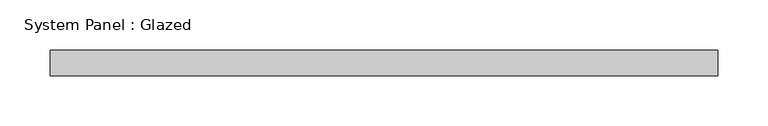
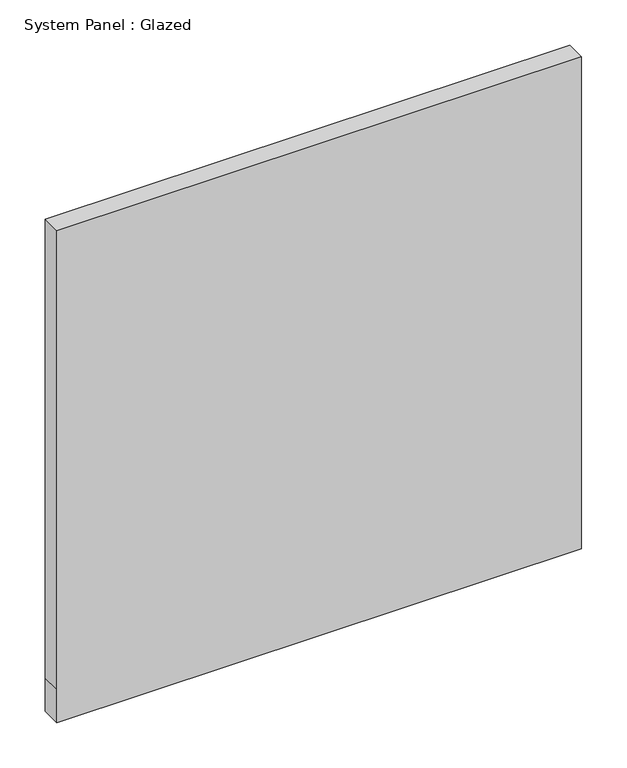
"""IFC4 building model written with IfcOpenShell, lengths in millimetres: plate geometry, System Panel : Glazed."""

from ifc_helpers import new_model, si_unit, frame, origin, place, context, project, spatial, polyline, outline, extrude, source, transform, mapped, element, save


def system_panel_glazed_81358e4c(model_context):
    return source(origin(), model_context, "Body", "SweptSolid", [
        extrude(outline(polyline([(0.0, -333.375), (0.0, 333.375), (44.45, 333.375), (660.9888769, 333.375), (660.9888769, -333.375), (44.45, -333.375), (0.0, -333.375)])), frame((0.0, 19.05, 0.0), z_axis=(0.0, 1.0, 0.0), x_axis=(0.0, 0.0, 1.0)), (0.0, 0.0, 1.0), 25.4),
    ])


if __name__ == "__main__":
    model = new_model("IFC4")
    model_context = context("Model", 3, world=origin())
    ifc_project = project(units=[si_unit("LENGTHUNIT", "METRE", prefix="MILLI")], contexts=[model_context])
    site = spatial("IfcSite", under=ifc_project)
    building = spatial("IfcBuilding", under=site)
    placement = place(None, origin())
    system_panel_glazed_shape = system_panel_glazed_81358e4c(model_context)
    element("IfcPlate", 1, ObjectType="System Panel : Glazed", at=placement, inside=building, context=model_context, shape_type="MappedRepresentation", body=[
        mapped(system_panel_glazed_shape, transform((0.0, 0.0, 0.0), x_axis=(1.0, 0.0, 0.0), y_axis=(0.0, 1.0, 0.0), z_axis=(0.0, 0.0, 1.0))),
    ])
    save(model, "model.ifc")

# Revit data of these elements
# Type "System Panel : Glazed"
#   Construction Type Id = "GSP4R"
#   Analytic Construction = "1/8 in Pilkington single glazing"
#   Visual Light Transmittance = 0.9
#   Solar Heat Gain Coefficient = 0.86
#   Heat Transfer Coefficient (U) = 1.18115 BTU/(h·ft²·°F)
#   Define Thermal Properties by = 1
# Element 1 (IfcPlate, "System Panel : Glazed")
#   Materials on its faces: "Glass"
# Materials
#   "Glass": class "Glass", colour RGB 0 128 192, transparency 0.75, Description = "Soda Lime Glass", Cost = 0
